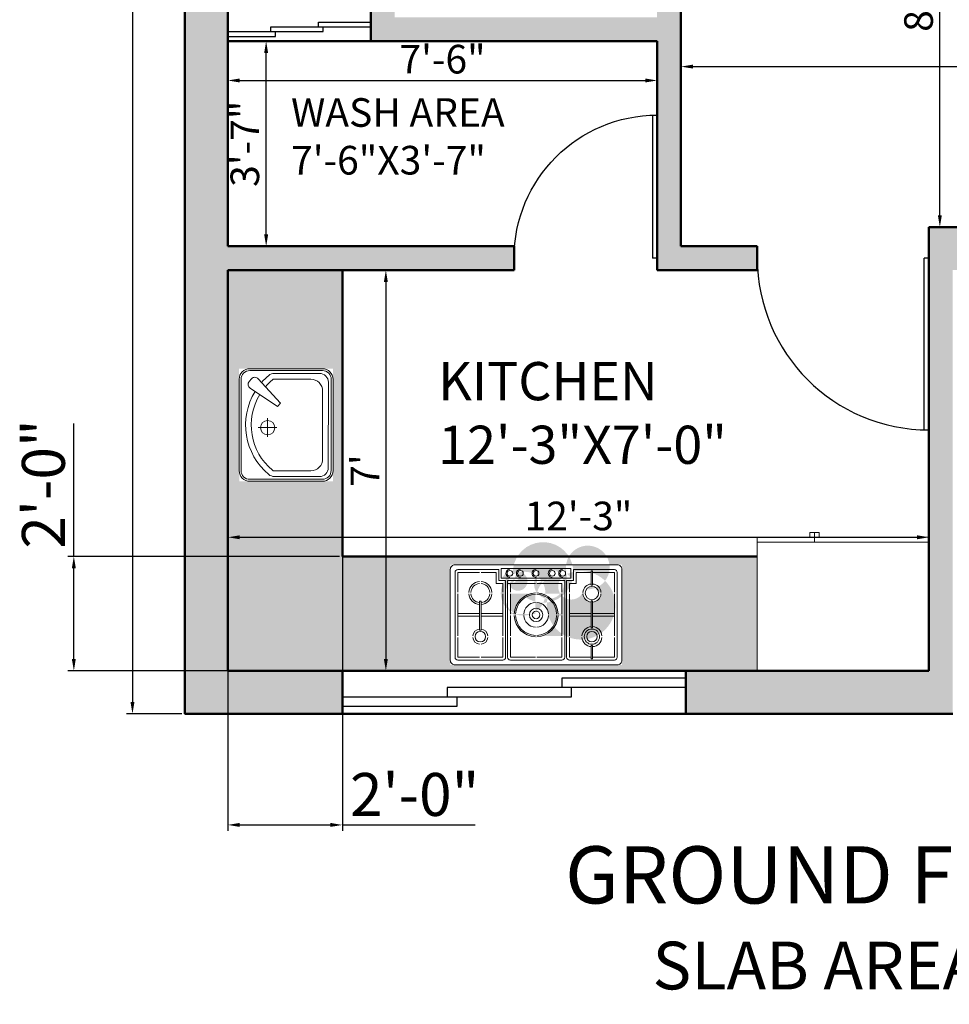
# Model space of a CAD drawing. Units: inches. Extents: x 3274 to 5176, y 1085 to 2172.
# Tile 11 of 16: x 4323 to 4517, y 1112 to 1319. Entities that reach past the tile are written whole.
import ezdxf

# ---------------------------------------------------------------- set-up
doc = ezdxf.new("R2010")
doc.units = ezdxf.units.IN
for name, color, linetype, lineweight in [('A-ANNO-DIMS', 2, 'Continuous', 18), ('A-ANNO-TEXT', 7, 'Continuous', 25), ('A-AREA-IDEN', 3, 'Continuous', 25), ('A-DOOR', 4, 'Continuous', 25), ('A-FLOR-FIXT', 8, 'Continuous', 18), ('A-FLOR-PATT', 252, 'Continuous', 13), ('A-GLAZ', 5, 'Continuous', 25), ('A-WALL', 7, 'Continuous', 50), ('A-WALL-PATT', 8, 'Continuous', 13)]:
    doc.layers.add(name, color=color, linetype=linetype, lineweight=lineweight)
doc.styles.get("Standard").update_dxf_attribs({"font": 'arial.ttf'})
doc.dimstyles.new('ISO-25', dxfattribs={"dimtxt": 9, "dimasz": 2.5, "dimexe": 1.25, "dimexo": 0.625, "dimtad": 1, "dimdec": 1, "dimlunit": 3, "dimtxsty": 'Standard', "dimcen": 2.5, "dimclrd": 4, "dimclre": 4, "dimclrt": 1, "dimadec": 0, "dimazin": 0, "dimtfac": 1, "dimtdec": 1, "dimtmove": 0, "dimatfit": 3, "dimfxl": 1, "dimarcsym": 0})

# ---------------------------------------------------------------- blocks, each defined once
blk = doc.blocks.new('2')
for p, q in [((0, 30), (0, 0)), ((1, 30), (1, 0)), ((0, 0), (1, 0))]:
    blk.add_line(p, q)
blk.add_arc((0, 0), 30, 0, 90)
blk = doc.blocks.new('1')
for p, q in [((0, 36), (0, 0)), ((1, 36), (1, 0)), ((0, 0), (1, 0))]:
    blk.add_line(p, q)
blk.add_arc((0, 0), 36, 0, 90)
blk = doc.blocks.new('*D7')
at = {"layer": 'A-ANNO-DIMS', "color": 0, "lineweight": -2, "transparency": 16777216}
for p, q in [((4356.56, 1533.35), (4344.93, 1533.35)), ((4346.18, 1530.85), (4346.18, 1175.85)), ((4356.56, 1173.35), (4344.93, 1173.35))]:
    blk.add_line(p, q, dxfattribs=at)
at = {"layer": 'A-ANNO-DIMS', "color": 0, "transparency": 16777216}
for points in [[(4345.77, 1530.85), (4346.6, 1530.85), (4346.18, 1533.35)], [(4345.77, 1175.85), (4346.6, 1175.85), (4346.18, 1173.35)]]:
    blk.add_solid(points, dxfattribs=at)
at = {"layer": 'Defpoints', "color": 0, "transparency": 16777216}
for p in [(4357.19, 1533.35), (4346.18, 1173.35), (4357.19, 1173.35)]:
    blk.add_point(p, dxfattribs=at)
at = {"layer": 'A-ANNO-DIMS', "color": 0, "transparency": 16777216, "insert": (4340.96, 1353.35), "char_height": 9, "attachment_point": 5, "rotation": 90}
blk.add_mtext("30'", dxfattribs=at)
blk = doc.blocks.new('STOVE')
for p, q in [((11.85, 19.7), (11.55, 19.7)), ((11.55, 16.92), (11.55, 19.7)), ((11.85, 16.92), (11.85, 19.7)), ((11.85, 16.92), (11.55, 16.92)), ((-11.85, 13.73), (-11.85, 7.62)), ((-11.85, 13.73), (-11.55, 13.73)), ((-11.55, 13.73), (-11.55, 7.62)), ((11.85, 13.23), (11.55, 13.23)), ((11.55, 13.23), (11.55, 7.57)), ((11.85, 13.23), (11.85, 7.57)), ((-11.85, 10.75), (-16.4, 10.75)), ((-7, 10.75), (-11.55, 10.75)), ((7, 10.75), (11.55, 10.75)), ((11.85, 10.75), (16.4, 10.75)), ((-11.85, 10.25), (-16.4, 10.25)), ((-7, 10.25), (-11.55, 10.25)), ((7, 10.25), (11.55, 10.25)), ((11.85, 10.25), (16.4, 10.25)), ((-11.85, 7.62), (-11.55, 7.62)), ((11.85, 7.57), (11.55, 7.57)), ((11.85, 4.28), (11.55, 4.28)), ((11.55, 4.28), (11.55, 1.3)), ((11.85, 4.28), (11.85, 1.3)), ((-7, 3.9), (-8.4, 3.9)), ((-7.8, 3.3), (-7.8, 1)), ((-6.4, 3.3), (-7.8, 3.3)), ((7.3, 2.8), (-7.3, 2.8)), ((-7.3, 2.8), (-7.3, 0.8)), ((-5.4, 3.9), (-6, 3.9)), ((-5.4, 3.9), (-0.15, 3.9)), ((0.15, 3.9), (5.4, 3.9)), ((6.4, 3.3), (7.8, 3.3)), ((7, 3.9), (8.4, 3.9)), ((7.3, 2.8), (7.3, 0.8)), ((7.8, 3.3), (7.8, 1)), ((8.4, 3.9), (8.4, 1.6)), ((7.3, 0.8), (-7.3, 0.8)), ((11.85, 1.3), (11.55, 1.3))]:
    blk.add_line(p, q)
for points in [[(-17, 21), (17, 21, -0.414214), (18, 20), (18, 1, -0.414214), (17, 0), (-17, 0, -0.414214), (-18, 1), (-18, 20, -0.414214)], [(6, 3.3), (-6, 3.3), (-6, 19.4, -0.414214), (-5.4, 20), (5.4, 20, -0.414214), (6, 19.4)]]:
    blk.add_lwpolyline(points, format="xyb", close=True)
for points in [[(-7.8, 1), (-16.4, 1, -0.414214), (-17, 1.6), (-17, 19.4, -0.414214), (-16.4, 20), (-7, 20, -0.414214), (-6.4, 19.4), (-6.4, 3.3)], [(6.4, 19.4, -0.414214), (7, 20), (16.4, 20, -0.414214), (17, 19.4), (17, 1.6, -0.414214), (16.4, 1), (7.8, 1)]]:
    blk.add_lwpolyline(points, format="xyb")
for points in [[(-16.4, 15.22), (-16.4, 19.4), (-11.85, 19.4)], [(-11.55, 19.4), (-7, 19.4), (-7, 15.22)], [(-5.4, 15.22), (-5.4, 19.4), (-0.15, 19.4)], [(0.15, 19.4), (5.4, 19.4), (5.4, 15.22)], [(6.4, 3.3), (6.4, 19.4)], [(7, 15.22), (7, 19.4), (11.55, 19.4)], [(11.85, 19.4), (16.4, 19.4), (16.4, 15.22)], [(-16.4, 6.08), (-16.4, 14.92)], [(-7, 14.92), (-7, 6.08)], [(-5.4, 10.65), (-5.4, 14.92)], [(5.4, 14.92), (5.4, 10.65)], [(7, 6.08), (7, 14.92)], [(16.4, 14.92), (16.4, 6.08)], [(-5.4, 6.08), (-5.4, 10.35)], [(5.4, 10.35), (5.4, 6.08)], [(-11.85, 1.6), (-16.4, 1.6), (-16.4, 5.77)], [(-7, 5.77), (-7, 3.9)], [(-5.4, 3.9), (-5.4, 5.77)], [(5.4, 5.77), (5.4, 3.9)], [(7, 3.9), (7, 5.77)], [(16.4, 5.77), (16.4, 1.6), (11.85, 1.6)], [(-8.4, 3.9), (-8.4, 1.6), (-11.55, 1.6)], [(11.55, 1.6), (8.4, 1.6)]]:
    blk.add_lwpolyline(points)
for centre, radius in [((11.7, 15.07), 1.6), ((-11.7, 15.07), 1.1), ((11.7, 15.07), 1.1), ((0, 10.5), 1.4), ((0, 10.5), 0.8), ((11.7, 5.93), 1.4), ((-5.49, 1.8), 0.6), ((-3.3, 1.8), 0.6), ((0, 1.8), 0.6), ((3.39, 1.8), 0.6), ((5.57, 1.8), 0.6)]:
    blk.add_circle(centre, radius)
for centre, radius, start, end in [((-11.7, 15.07), 1.6, 95.3794, 174.6206), ((-11.7, 15.07), 1.6, 5.3794, 84.6206), ((11.7, 15.07), 2.1, 94.096, 175.904), ((11.7, 15.07), 2.1, 4.096, 85.904), ((-11.7, 15.07), 1.6, 185.3794, 264.6206), ((-11.7, 15.07), 1.6, 275.3794, 354.6206), ((0, 10.5), 4.6, 91.8687, 178.1313), ((0, 10.5), 4.3, 91.9991, 178.0009), ((0, 10.5), 4.6, 1.8687, 88.1313), ((0, 10.5), 4.3, 1.9991, 88.0009), ((11.7, 15.07), 2.1, 184.096, 265.904), ((11.7, 15.07), 2.1, 274.096, 355.904), ((0, 10.5), 2.6, 93.3074, 176.6926), ((0, 10.5), 2.6, 3.3074, 86.6926), ((0, 10.5), 4.6, 181.8687, 268.1313), ((0, 10.5), 4.3, 181.9991, 268.0009), ((0, 10.5), 2.6, 183.3074, 266.6926), ((0, 10.5), 4.6, 271.8687, 358.1313), ((0, 10.5), 4.3, 271.9991, 358.0009), ((0, 10.5), 2.6, 273.3074, 356.6926), ((-11.7, 5.93), 2.4, 93.5833, 176.4167), ((-11.7, 5.93), 2.4, 3.5833, 86.4167), ((-11.7, 5.93), 2, 94.3012, 175.6988), ((-11.7, 5.93), 2, 4.3012, 85.6988), ((11.7, 5.93), 1.9, 94.5281, 175.4719), ((11.7, 5.93), 1.9, 4.5281, 85.4719), ((-11.7, 5.93), 2.4, 183.5833, 266.4167), ((-11.7, 5.93), 2, 184.3012, 265.6988), ((-11.7, 5.93), 2.4, 273.5833, 356.4167), ((-11.7, 5.93), 2, 274.3012, 355.6988), ((11.7, 5.93), 1.9, 184.5281, 265.4719), ((11.7, 5.93), 1.9, 274.5281, 355.4719), ((-5.49, 1.8), 0.846, 89.9979, 270), ((-3.3, 1.8), 0.846, 89.9979, 270), ((0, 1.8), 0.846, 89.9979, 270), ((3.39, 1.8), 0.846, 89.9979, 270), ((5.57, 1.8), 0.846, 89.9979, 270)]:
    blk.add_arc(centre, radius, start, end)
blk = doc.blocks.new('Refrigerator-2 door - 36 in top')
for p, q in [((0, -26.999999), (36, -26.999999)), ((11, -27.999999), (11, -28.999999)), ((12, -26.999999), (12, -28.999999)), ((13, -28.999999), (13, -27.999999)), ((11, -28.999999), (13, -28.999999))]:
    blk.add_line(p, q)
blk.add_lwpolyline([(0, -27.999999), (0, 0), (36, 0), (36, -27.999999)], close=True)
blk = doc.blocks.new('*D73')
at = {"layer": 'A-ANNO-DIMS', "color": 0, "lineweight": -2, "transparency": 16777216}
for p, q in [((4366.81, 1314.35), (4375.46, 1314.35)), ((4374.21, 1273.85), (4374.21, 1311.85)), ((4366.81, 1271.35), (4375.46, 1271.35))]:
    blk.add_line(p, q, dxfattribs=at)
at = {"layer": 'A-ANNO-DIMS', "color": 0, "transparency": 16777216}
for points in [[(4373.79, 1311.85), (4374.63, 1311.85), (4374.21, 1314.35)], [(4373.79, 1273.85), (4374.63, 1273.85), (4374.21, 1271.35)]]:
    blk.add_solid(points, dxfattribs=at)
at = {"layer": 'Defpoints', "color": 0, "transparency": 16777216}
for p in [(4366.19, 1314.35), (4374.21, 1314.35), (4366.19, 1271.35)]:
    blk.add_point(p, dxfattribs=at)
at = {"layer": 'A-ANNO-DIMS', "color": 0, "transparency": 16777216, "insert": (4370.52, 1292.85), "char_height": 6, "attachment_point": 5, "rotation": 90}
blk.add_mtext('3\'-7"', dxfattribs=at)
blk = doc.blocks.new('*D74')
at = {"layer": 'A-ANNO-DIMS', "color": 0, "lineweight": -2, "transparency": 16777216}
for p, q in [((4366.19, 1313.73), (4366.19, 1304.86)), ((4456.19, 1313.73), (4456.19, 1304.86)), ((4368.69, 1306.11), (4453.69, 1306.11))]:
    blk.add_line(p, q, dxfattribs=at)
at = {"layer": 'A-ANNO-DIMS', "color": 0, "transparency": 16777216}
for points in [[(4368.69, 1306.53), (4368.69, 1305.7), (4366.19, 1306.11)], [(4453.69, 1306.53), (4453.69, 1305.7), (4456.19, 1306.11)]]:
    blk.add_solid(points, dxfattribs=at)
at = {"layer": 'Defpoints', "color": 0, "transparency": 16777216}
for p in [(4366.19, 1314.35), (4456.19, 1314.35), (4456.19, 1306.11)]:
    blk.add_point(p, dxfattribs=at)
at = {"layer": 'A-ANNO-DIMS', "color": 0, "transparency": 16777216, "insert": (4411.19, 1309.8), "char_height": 6, "attachment_point": 5}
blk.add_mtext('7\'-6"', dxfattribs=at)
blk = doc.blocks.new('*D75')
at = {"layer": 'A-ANNO-DIMS', "color": 0, "lineweight": -2, "transparency": 16777216}
for p, q in [((4390.81, 1266.35), (4400.56, 1266.35)), ((4399.31, 1263.85), (4399.31, 1184.85)), ((4390.81, 1182.35), (4400.56, 1182.35))]:
    blk.add_line(p, q, dxfattribs=at)
at = {"layer": 'A-ANNO-DIMS', "color": 0, "transparency": 16777216}
for points in [[(4398.89, 1263.85), (4399.73, 1263.85), (4399.31, 1266.35)], [(4398.89, 1184.85), (4399.73, 1184.85), (4399.31, 1182.35)]]:
    blk.add_solid(points, dxfattribs=at)
at = {"layer": 'Defpoints', "color": 0, "transparency": 16777216}
for p in [(4390.19, 1266.35), (4390.19, 1182.35), (4399.31, 1182.35)]:
    blk.add_point(p, dxfattribs=at)
at = {"layer": 'A-ANNO-DIMS', "color": 0, "transparency": 16777216, "insert": (4395.69, 1224.35), "char_height": 6, "attachment_point": 5, "rotation": 90}
blk.add_mtext("7'", dxfattribs=at)
blk = doc.blocks.new('*D76')
at = {"layer": 'A-ANNO-DIMS', "color": 0, "lineweight": -2, "transparency": 16777216}
for p, q in [((4366.19, 1209.19), (4366.19, 1211.6)), ((4368.69, 1210.35), (4510.69, 1210.35)), ((4513.19, 1209.19), (4513.19, 1211.6))]:
    blk.add_line(p, q, dxfattribs=at)
at = {"layer": 'A-ANNO-DIMS', "color": 0, "transparency": 16777216}
for points in [[(4368.69, 1210.77), (4368.69, 1209.94), (4366.19, 1210.35)], [(4510.69, 1210.77), (4510.69, 1209.94), (4513.19, 1210.35)]]:
    blk.add_solid(points, dxfattribs=at)
at = {"layer": 'Defpoints', "color": 0, "transparency": 16777216}
for p in [(4513.19, 1210.35), (4366.19, 1208.57), (4513.19, 1208.57)]:
    blk.add_point(p, dxfattribs=at)
at = {"layer": 'A-ANNO-DIMS', "color": 0, "transparency": 16777216, "insert": (4439.69, 1214.04), "char_height": 6, "attachment_point": 5}
blk.add_mtext('12\'-3"', dxfattribs=at)
blk = doc.blocks.new('*D81')
at = {"layer": 'A-ANNO-DIMS', "color": 0, "lineweight": -2, "transparency": 16777216}
for p, q in [((4461.19, 1312.95), (4461.19, 1307.77)), ((4708.19, 1312.95), (4708.19, 1307.77)), ((4463.69, 1309.02), (4705.69, 1309.02))]:
    blk.add_line(p, q, dxfattribs=at)
at = {"layer": 'A-ANNO-DIMS', "color": 0, "transparency": 16777216}
for points in [[(4463.69, 1309.44), (4463.69, 1308.61), (4461.19, 1309.02)], [(4705.69, 1309.44), (4705.69, 1308.61), (4708.19, 1309.02)]]:
    blk.add_solid(points, dxfattribs=at)
at = {"layer": 'Defpoints', "color": 0, "transparency": 16777216}
for p in [(4461.19, 1313.57), (4708.19, 1313.57), (4708.19, 1309.02)]:
    blk.add_point(p, dxfattribs=at)
at = {"layer": 'A-ANNO-DIMS', "color": 0, "transparency": 16777216, "insert": (4584.69, 1312.71), "char_height": 6, "attachment_point": 5}
blk.add_mtext('20\'-7"', dxfattribs=at)
blk = doc.blocks.new('*D82')
at = {"layer": 'A-ANNO-DIMS', "color": 0, "lineweight": -2, "transparency": 16777216}
for p, q in [((4513.81, 1375.35), (4516.72, 1375.35)), ((4515.47, 1277.85), (4515.47, 1372.85)), ((4513.81, 1275.35), (4516.72, 1275.35))]:
    blk.add_line(p, q, dxfattribs=at)
at = {"layer": 'A-ANNO-DIMS', "color": 0, "transparency": 16777216}
for points in [[(4515.05, 1372.85), (4515.88, 1372.85), (4515.47, 1375.35)], [(4515.05, 1277.85), (4515.88, 1277.85), (4515.47, 1275.35)]]:
    blk.add_solid(points, dxfattribs=at)
at = {"layer": 'Defpoints', "color": 0, "transparency": 16777216}
for p in [(4513.19, 1375.35), (4515.47, 1375.35), (4513.19, 1275.35)]:
    blk.add_point(p, dxfattribs=at)
at = {"layer": 'A-ANNO-DIMS', "color": 0, "transparency": 16777216, "insert": (4511.78, 1325.35), "char_height": 6, "attachment_point": 5, "rotation": 90}
blk.add_mtext('8\'-4"', dxfattribs=at)
blk = doc.blocks.new('WIN-30')
for p, q in [((4375.19, 1317.35), (4396.19, 1317.35)), ((4375.19, 1316.35), (4375.19, 1317.35)), ((4385.19, 1318.35), (4396.19, 1318.35)), ((4385.19, 1317.35), (4385.19, 1318.35)), ((4386.19, 1316.35), (4386.19, 1317.35)), ((4366.19, 1316.35), (4386.19, 1316.35)), ((4366.19, 1315.35), (4376.19, 1315.35)), ((4376.19, 1315.35), (4376.19, 1316.35))]:
    blk.add_line(p, q)
blk = doc.blocks.new('WIN-72')
for p, q in [((4462.19, 1180.85), (4436.19, 1180.85)), ((4436.19, 1180.85), (4436.19, 1178.85)), ((4462.19, 1178.85), (4412.19, 1178.85)), ((4412.19, 1178.85), (4412.19, 1176.85)), ((4438.19, 1178.85), (4438.19, 1176.85)), ((4438.19, 1176.85), (4390.19, 1176.85)), ((4414.19, 1176.85), (4414.19, 1174.85)), ((4414.19, 1174.85), (4390.19, 1174.85))]:
    blk.add_line(p, q)
blk = doc.blocks.new('SINK-KITCHEN')
at = {"transparency": 33554687}
for points in [[(4388.24, 1243.45, 0.414214), (4386.01, 1245.69), (4370.78, 1245.67, 0.414214), (4368.55, 1243.47), (4368.57, 1224.32, 0.414214), (4370.77, 1222.1), (4386.01, 1222.1, 0.414214), (4388.24, 1224.33), (4388.24, 1243.45)], [(4387.87, 1243.45, 0.414214), (4386.01, 1245.3), (4370.78, 1245.3, 0.414214), (4368.94, 1243.47), (4368.94, 1224.32, 0.414214), (4370.77, 1222.5), (4386.01, 1222.5, 0.414214), (4387.84, 1224.33), (4387.87, 1243.45)], [(4371.89, 1240.94, 0.371519), (4374.75, 1223.51, 0.175764), (4375.92, 1223.1), (4385.42, 1223.08, 0.414214), (4387.24, 1224.93), (4387.27, 1242.85, 0.414214), (4385.41, 1244.69), (4375.92, 1244.69, 0.175764), (4374.75, 1244.27, 0.038632), (4373.27, 1242.81)], [(4372.88, 1240.28, 0.370401), (4375.51, 1224.41, 0.175764), (4375.92, 1224.28), (4383.57, 1224.28, 0.414214), (4386.06, 1226.79), (4386.06, 1241, 0.414214), (4383.55, 1243.51), (4375.92, 1243.51, 0.175764), (4375.51, 1243.36, 0.038512), (4374.06, 1241.92)]]:
    blk.add_lwpolyline(points, format="xyb", dxfattribs=at)
blk.add_lwpolyline([(4371.14, 1243.58), (4370.66, 1243, 0.463205), (4370.87, 1241.61), (4376.59, 1237.78), (4377.2, 1238.48), (4372.56, 1243.56, 0.4637)], format="xyb", close=True, dxfattribs=at)
for points in [[(4374.51, 1231.4), (4374.51, 1235.3)], [(4372.56, 1233.35), (4376.46, 1233.35)]]:
    blk.add_lwpolyline(points, dxfattribs=at)
blk.add_circle((4374.52, 1233.34), 1.5, dxfattribs=at)
blk = doc.blocks.new('*D150')
at = {"layer": 'A-ANNO-DIMS', "color": 4, "lineweight": -2, "transparency": 16777216}
for p, q in [((4366.19, 1265.73), (4366.19, 1148.8)), ((4390.19, 1265.73), (4390.19, 1148.8)), ((4368.69, 1150.05), (4387.69, 1150.05)), ((4390.19, 1150.05), (4418.01, 1150.05))]:
    blk.add_line(p, q, dxfattribs=at)
at = {"layer": 'A-ANNO-DIMS', "color": 4, "transparency": 16777216}
for points in [[(4368.69, 1150.47), (4368.69, 1149.64), (4366.19, 1150.05)], [(4387.69, 1150.47), (4387.69, 1149.64), (4390.19, 1150.05)]]:
    blk.add_solid(points, dxfattribs=at)
at = {"layer": 'Defpoints', "color": 0, "transparency": 16777216}
for p in [(4366.19, 1266.35), (4390.19, 1266.35), (4390.19, 1150.05)]:
    blk.add_point(p, dxfattribs=at)
at = {"layer": 'A-ANNO-DIMS', "color": 1, "transparency": 16777216, "insert": (4405.35, 1155.27), "char_height": 9, "attachment_point": 5}
blk.add_mtext('2\'-0"', dxfattribs=at)
blk = doc.blocks.new('*D151')
at = {"layer": 'A-ANNO-DIMS', "color": 4, "lineweight": -2, "transparency": 16777216}
for p, q in [((4333.89, 1206.35), (4333.89, 1234.18)), ((4389.56, 1206.35), (4332.64, 1206.35)), ((4333.89, 1184.85), (4333.89, 1203.85)), ((4389.56, 1182.35), (4332.64, 1182.35))]:
    blk.add_line(p, q, dxfattribs=at)
at = {"layer": 'A-ANNO-DIMS', "color": 4, "transparency": 16777216}
for points in [[(4333.47, 1203.85), (4334.3, 1203.85), (4333.89, 1206.35)], [(4333.47, 1184.85), (4334.3, 1184.85), (4333.89, 1182.35)]]:
    blk.add_solid(points, dxfattribs=at)
at = {"layer": 'Defpoints', "color": 0, "transparency": 16777216}
for p in [(4333.89, 1206.35), (4390.19, 1206.35), (4390.19, 1182.35)]:
    blk.add_point(p, dxfattribs=at)
at = {"layer": 'A-ANNO-DIMS', "color": 1, "transparency": 16777216, "insert": (4328.67, 1221.52), "char_height": 9, "attachment_point": 5, "rotation": 90}
blk.add_mtext('2\'-0"', dxfattribs=at)

msp = doc.modelspace()

# ---------------------------------------------------------------- hatches: boundary and pattern name
at = {"layer": 'A-FLOR-PATT'}
h = msp.add_hatch(color=256, dxfattribs=at)
h.dxf.hatch_style = 1
h.paths.add_polyline_path([(4366.19, 1182.35), (4477.19, 1182.35), (4477.19, 1206.35), (4390.19, 1206.35), (4390.19, 1266.35), (4366.19, 1266.35)])
h.paths.add_polyline_path([(4368.57, 1222.1), (4368.54, 1245.67), (4388.24, 1245.7), (4388.24, 1222.1)], flags=16)
h.paths.add_polyline_path([(4368.94, 1222.5), (4368.94, 1245.3), (4387.87, 1245.3), (4387.84, 1222.5)], flags=0)
h.paths.add_polyline_path([(4371.89, 1240.93), (4371.33, 1242.2, -1.098558), (4372.49, 1243.63), (4373.26, 1242.79, -0.038991), (4374.75, 1244.26, -0.176171), (4375.92, 1244.69), (4387.27, 1244.69), (4387.24, 1223.07), (4375.26, 1223.1, -0.384983)], flags=0)
h.paths.add_polyline_path([(4373.02, 1233.35, -0.996132), (4376.02, 1233.34, -0.416486), (4374.51, 1231.84), (4374.51, 1233.35)], flags=0)
h.paths.add_polyline_path([(4412.82, 1204.59), (4448.82, 1204.59), (4448.82, 1183.59), (4412.82, 1183.59)], flags=16)
h.paths.add_polyline_path([(4413.82, 1203.59), (4423.02, 1203.59), (4423.52, 1203.6), (4423.52, 1203.79), (4442.67, 1203.79), (4442.67, 1203.59), (4447.82, 1203.59), (4447.82, 1184.59), (4437.82, 1184.59), (4425.42, 1184.59), (4413.82, 1184.59)], flags=0)
h.paths.add_polyline_path([(4425.34, 1201.94, -0.414214), (4424.49, 1202.79), (4423.82, 1202.11), (4423.82, 1201.79)], flags=16)
h.paths.add_polyline_path([(4426.68, 1202.79), (4426.01, 1200.69), (4427.52, 1201.94, -0.414214)], flags=16)
h.paths.add_polyline_path([(4432.08, 1189.67), (4436.22, 1189.67), (4436.22, 1193.94), (4435.42, 1193.94, -0.326254)], flags=16)
h.paths.add_polyline_path([(4437.22, 1202.96), (4437.22, 1201.29), (4438.62, 1201.29), (4437.24, 1202.79, -3.134619), (4441.36, 1199.45, -0.740447), (4443.92, 1198.67), (4444.4, 1198.96, -0.460532), (4442.52, 1196.77), (4442.67, 1196.69), (4442.67, 1197.02), (4442.37, 1197.02), (4442.37, 1196.77, -0.391251), (4440.62, 1198.67), (4440.58, 1198.52), (4440.88, 1198.52), (4440.88, 1198.82), (4440.63, 1198.82, -1.371894), (4436.89, 1202.45, -4.789177), (4433.3, 1197.96, -0.241151), (4435.42, 1194.34), (4436.22, 1194.34), (4436.22, 1198.52), (4430.97, 1198.52), (4430.97, 1198.39, -0.424384), (4435.94, 1202.07, -1.499909)], flags=16)
h.paths.add_polyline_path([(4425.34, 1202.19, -0.243811), (4430.22, 1202.79, -0.490314), (4430.97, 1203.37), (4430.97, 1200.69), (4434.21, 1201.94, -1), (4434.21, 1203.64, -3.06951), (4430.82, 1202.19), (4431.26, 1202.07, -3.176421), (4425.94, 1202.79, -4.490619), (4428.37, 1197.98, 0.248869), (4426.22, 1194.24), (4426.52, 1194.24, -0.6999), (4427.73, 1202.23, -3.209262), (4428.12, 1202.79, -2.374197), (4425.34, 1202.19), (4423.59, 1201.29)], flags=16)
h.paths.add_polyline_path([(4430.67, 1198.52), (4425.42, 1198.52), (4425.42, 1194.24), (4430.67, 1194.24)], flags=16)
at = {"layer": 'A-WALL-PATT'}
h = msp.add_hatch(color=256, dxfattribs=at)
h.dxf.hatch_style = 1
h.paths.add_polyline_path([(4717.19, 1533.35), (4357.19, 1533.35), (4357.19, 1173.35), (4390.19, 1173.35), (4390.19, 1182.35), (4366.19, 1182.35), (4366.19, 1266.35), (4426.19, 1266.35), (4426.19, 1271.35), (4366.19, 1271.35), (4366.19, 1375.35), (4426.19, 1375.35), (4426.19, 1380.35), (4366.19, 1380.35), (4366.19, 1524.35), (4708.19, 1524.35), (4708.19, 1380.35), (4578.19, 1380.35), (4578.19, 1375.35), (4708.19, 1375.35), (4708.19, 1275.35), (4640.19, 1275.35), (4640.19, 1266.35), (4708.19, 1266.35), (4708.19, 1182.35), (4666.19, 1182.35), (4666.19, 1173.35), (4717.19, 1173.35)])
h.paths.add_polyline_path([(4461.19, 1375.35), (4477.19, 1375.35), (4477.19, 1380.35), (4456.19, 1380.35), (4456.19, 1319.35), (4401.19, 1319.35), (4401.19, 1339.35), (4396.19, 1339.35), (4396.19, 1314.35), (4456.19, 1314.35), (4456.19, 1266.35), (4477.19, 1266.35), (4477.19, 1271.35), (4461.19, 1271.35)], flags=17)
h.paths.add_polyline_path([(4518.19, 1483.35), (4536.19, 1483.35), (4536.19, 1488.35), (4513.19, 1488.35), (4513.19, 1375.35), (4536.19, 1375.35), (4536.19, 1380.35), (4518.19, 1380.35), (4518.19, 1418.35), (4548.19, 1418.35), (4548.19, 1423.35), (4518.19, 1423.35)], flags=17)
h.paths.add_polyline_path([(4583.19, 1488.35), (4560.19, 1488.35), (4560.19, 1483.35), (4578.19, 1483.35), (4578.19, 1416.35), (4583.19, 1416.35)], flags=17)
h.paths.add_polyline_path([(4518.19, 1266.35), (4523.19, 1266.35), (4523.19, 1275.35), (4513.19, 1275.35), (4513.19, 1182.35), (4462.19, 1182.35), (4462.19, 1173.35), (4518.19, 1173.35)], flags=17)
h.paths.add_polyline_path([(4580.19, 1275.35), (4571.19, 1275.35), (4571.19, 1270.85), (4571.19, 1266.35), (4580.19, 1266.35)], flags=17)
h.paths.add_polyline_path([(4594.19, 1182.35), (4578.19, 1182.35), (4578.19, 1173.35), (4594.19, 1173.35)], flags=17)
h.paths.add_polyline_path([(4573.24, 1316.29), (4647.44, 1316.29), (4647.44, 1346.14), (4573.24, 1346.14)], flags=25)
h.paths.add_polyline_path([(4529.43, 1453), (4568.61, 1453), (4568.61, 1475.39), (4529.43, 1475.39)], flags=25)
h.paths.add_polyline_path([(4619, 1443.76), (4687.39, 1443.76), (4687.39, 1473.61), (4619, 1473.61)], flags=25)
h.paths.add_polyline_path([(4527.67, 1497.04), (4569.64, 1497.04), (4569.64, 1519.43), (4527.67, 1519.43)], flags=25)
h.paths.add_polyline_path([(4407.08, 1443.76), (4475.47, 1443.76), (4475.47, 1473.61), (4407.08, 1473.61)], flags=25)

# ---------------------------------------------------------------- linework, layer by layer
at = {"layer": 'A-WALL'}
for p, q in [((4366.19, 1271.35), (4366.19, 1375.35)), ((4461.19, 1271.35), (4461.19, 1375.35)), ((4396.19, 1314.35), (4396.19, 1339.35)), ((4366.19, 1314.35), (4456.19, 1314.35)), ((4456.19, 1266.35), (4456.19, 1314.35)), ((4513.19, 1182.35), (4513.19, 1275.35)), ((4513.19, 1275.35), (4523.19, 1275.35)), ((4366.19, 1271.35), (4426.19, 1271.35)), ((4426.19, 1266.35), (4426.19, 1271.35)), ((4461.19, 1271.35), (4477.19, 1271.35)), ((4477.19, 1266.35), (4477.19, 1271.35)), ((4366.19, 1182.35), (4366.19, 1266.35)), ((4366.19, 1266.35), (4426.19, 1266.35)), ((4390.19, 1206.35), (4390.19, 1266.35)), ((4456.19, 1266.35), (4477.19, 1266.35)), ((4477.19, 1206.35), (4390.19, 1206.35)), ((4513.19, 1182.35), (4366.19, 1182.35)), ((4390.19, 1182.35), (4390.19, 1173.35)), ((4462.19, 1182.35), (4462.19, 1173.35))]:
    msp.add_line(p, q, dxfattribs=at)
msp.add_lwpolyline([(4518.19, 1173.35), (4357.19, 1173.35), (4357.19, 1533.35), (4717.19, 1533.35), (4717.19, 1173.35), (4578.19, 1173.35)], dxfattribs=at)

# ---------------------------------------------------------------- block references
at = {"layer": 'A-DOOR', "xscale": -1}
msp.add_blockref('2', (4456.19, 1268.85), dxfattribs=at)
at = {"layer": 'A-DOOR', "rotation": 180}
msp.add_blockref('1', (4513.19, 1268.85), dxfattribs=at)
at = {"layer": 'A-FLOR-FIXT'}
msp.add_blockref('SINK-KITCHEN', (0, 0), dxfattribs=at)
at = {"layer": 'A-FLOR-FIXT', "xscale": -1, "rotation": 180}
for name, p in [('Refrigerator-2 door - 36 in top', (4477.19, 1182.35)), ('STOVE', (4430.82, 1204.59))]:
    msp.add_blockref(name, p, dxfattribs=at)
at = {"layer": 'A-GLAZ'}
for name in ['WIN-30', 'WIN-72']:
    msp.add_blockref(name, (0, 0), dxfattribs=at)

# ---------------------------------------------------------------- texts
at = {"layer": 'A-ANNO-TEXT', "insert": (4436.88, 1145.58), "char_height": 12, "attachment_point": 1}
msp.add_mtext_dynamic_manual_height_columns('GROUND FLOOR PLAN\\P{\\H0.83333x;      SLAB AREA-900Sq.ft}', width=202.3193, gutter_width=30, heights=[0], dxfattribs=at)
at = {"layer": 'A-AREA-IDEN', "attachment_point": 1}
for s, insert, char_height in [('WASH AREA\\P7\'-6"X3\'-7"', (4379.43, 1302.4), 6), ('KITCHEN\\P12\'-3"X7\'-0"', (4410.29, 1247.08), 8)]:
    msp.add_mtext_dynamic_manual_height_columns(s, width=58.0121, gutter_width=30, heights=[0], dxfattribs=dict(at, insert=insert, char_height=char_height))

# ---------------------------------------------------------------- dimensions: what is measured, and where the dimension line sits
at = {"layer": 'A-ANNO-DIMS'}
for base, p1, p2, override, picture, middle in [((4346.18, 1173.35), (4357.19, 1533.35), (4357.19, 1173.35), {"dimclrd": 0, "dimclre": 0, "dimclrt": 0}, '*D7', (4340.96, 1353.35)), ((4515.47, 1375.35), (4513.19, 1275.35), (4513.19, 1375.35), {"dimtxt": 6, "dimclrd": 0, "dimclre": 0, "dimclrt": 0}, '*D82', (4511.78, 1325.35)), ((4374.21, 1314.35), (4366.19, 1271.35), (4366.19, 1314.35), {"dimtxt": 6, "dimclrd": 0, "dimclre": 0, "dimclrt": 0}, '*D73', (4370.52, 1292.85)), ((4399.31, 1182.35), (4390.19, 1266.35), (4390.19, 1182.35), {"dimtxt": 6, "dimclrd": 0, "dimclre": 0, "dimclrt": 0}, '*D75', (4395.69, 1224.35)), ((4333.89, 1206.35), (4390.19, 1182.35), (4390.19, 1206.35), {"dimdec": 1, "dimlfac": 1, "dimrnd": 0, "dimzin": 1, "dimdsep": 46, "dimlunit": 4, "dimfrac": 2}, '*D151', (4328.67, 1221.52))]:
    dim = msp.add_linear_dim(base=base, p1=p1, p2=p2, angle=90, dimstyle='ISO-25', override=override, dxfattribs=at)
    dim.commit()
    dim.dimension.update_dxf_attribs({"geometry": picture, "text_midpoint": middle})
for base, p1, p2, override, picture, middle in [((4708.19, 1309.02), (4461.19, 1313.57), (4708.19, 1313.57), {"dimtxt": 6, "dimclrd": 0, "dimclre": 0, "dimclrt": 0}, '*D81', (4584.69, 1312.71)), ((4456.19, 1306.11), (4366.19, 1314.35), (4456.19, 1314.35), {"dimtxt": 6, "dimclrd": 0, "dimclre": 0, "dimclrt": 0}, '*D74', (4411.19, 1309.8)), ((4390.19, 1150.05), (4366.19, 1266.35), (4390.19, 1266.35), {"dimdec": 1, "dimlfac": 1, "dimrnd": 0, "dimzin": 1, "dimdsep": 46, "dimlunit": 4, "dimfrac": 2}, '*D150', (4405.35, 1155.27)), ((4513.19, 1210.35), (4366.19, 1208.57), (4513.19, 1208.57), {"dimtxt": 6, "dimclrd": 0, "dimclre": 0, "dimclrt": 0}, '*D76', (4439.69, 1214.04))]:
    dim = msp.add_linear_dim(base=base, p1=p1, p2=p2, dimstyle='ISO-25', override=override, dxfattribs=at)
    dim.commit()
    dim.dimension.update_dxf_attribs({"geometry": picture, "text_midpoint": middle})

doc.saveas('drawing.dxf')
